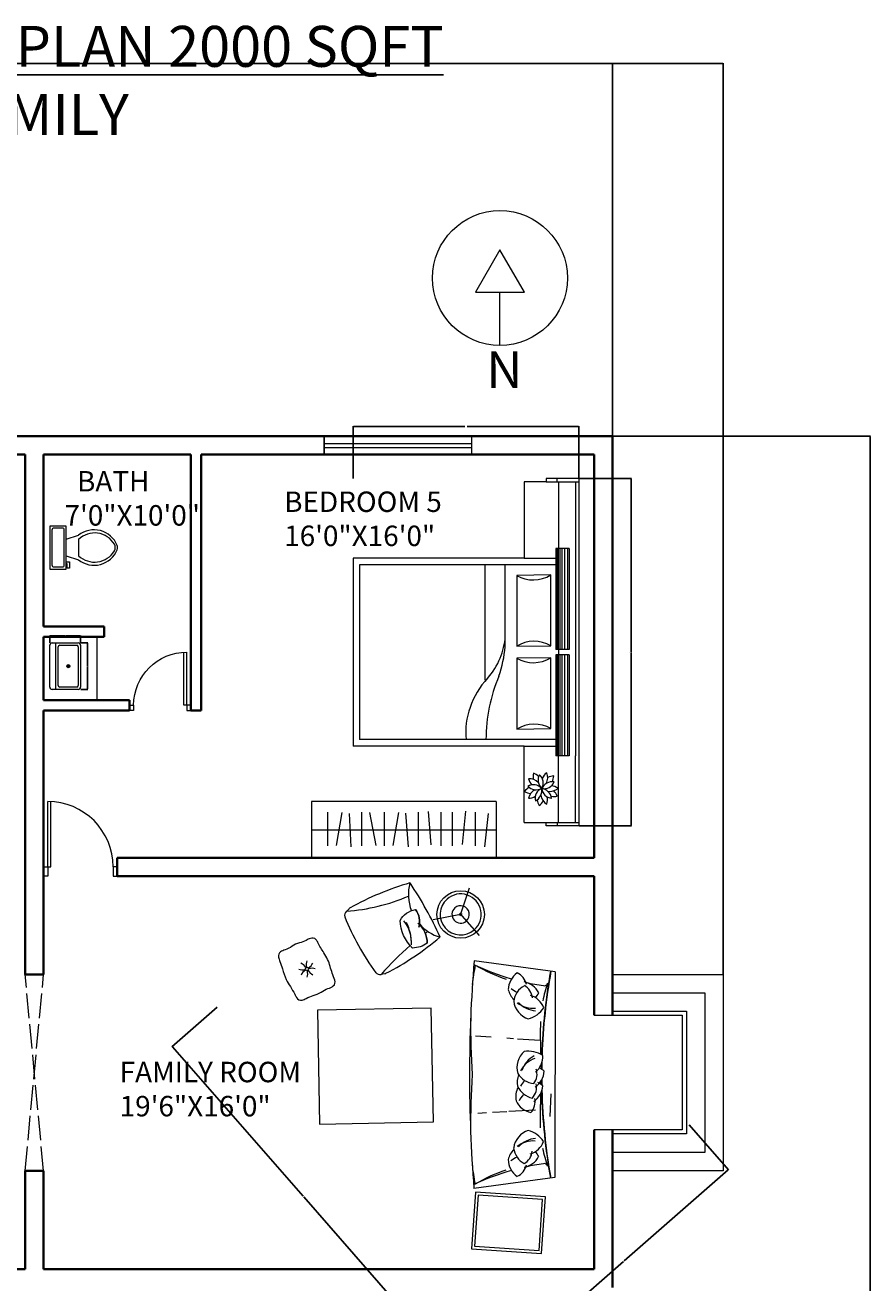
# Model space of a CAD drawing. Units: inches. Extents: x 4602 to 5612, y 5125 to 6591.
# Tile 6 of 6: x 5199 to 5612, y 5977 to 6591. Entities that reach past the tile are written whole.
import ezdxf

# ---------------------------------------------------------------- set-up
doc = ezdxf.new("R2010")
doc.units = ezdxf.units.IN
doc.linetypes.add('ACAD_ISO02W100', pattern=[15, 12, -3])
for name, color, linetype, lineweight in [('A-ANNO-DIMS', 2, 'Continuous', 18), ('A-ANNO-SYMB', 7, 'Continuous', 18), ('A-ANNO-TEXT', 7, 'Continuous', 25), ('A-AREA-IDEN', 7, 'Continuous', 18), ('A-DOOR', 4, 'Continuous', 18), ('A-FLOR-CASE', 9, 'Continuous', 18), ('A-FLOR-EDGE', 7, 'Continuous', 18), ('A-FLOR-FIXT', 8, 'Continuous', 18), ('A-FURN', 8, 'Continuous', 13), ('A-GLAZ', 4, 'Continuous', 18), ('A-WALL', 7, 'Continuous', 35), ('A-WALL-OVHD', 8, 'ACAD_ISO02W100', 13)]:
    doc.layers.add(name, color=color, linetype=linetype, lineweight=lineweight)
doc.styles.add('ATTR', font='romans.shx', dxfattribs={"width": 0.8, "height": 1.075})
doc.styles.get("Standard").update_dxf_attribs({"font": 'arial.ttf'})
doc.dimstyles.get("Standard").update_dxf_attribs({"dimtxt": 0.18, "dimasz": 0.18, "dimexe": 0.18, "dimexo": 0.0625, "dimgap": 0.09, "dimtad": 0, "dimtih": 1, "dimtoh": 1, "dimdec": 4, "dimzin": 0, "dimdsep": 46, "dimtxsty": 'Standard', "dimcen": 0.09, "dimadec": 0, "dimazin": 0, "dimtfac": 1, "dimtdec": 4, "dimtofl": 0, "dimtmove": 0, "dimatfit": 3, "dimfxl": 1, "dimtolj": 1, "dimtzin": 0, "dimarcsym": 0})

# ---------------------------------------------------------------- blocks, each defined once
blk = doc.blocks.new('A$C25213C04')
for p, q in [((2063, 2927, 1584), (1415, 2360, 1584)), ((2063, 2927, 1584), (3697, 1495, 1584)), ((961, 2561), (805, 2831)), ((961, 2590), (805, 2320)), ((936, 2575), (1248, 2575)), ((2506, 2330, 1584), (2338, 2162, 1584)), ((2306, 2131, 1584), (2256, 2081, 1584)), ((3178, 1881), (3005, 2048)), ((2140, 1966, 1584), (2022, 1849, 1584)), ((3026, 1811, 1584), (2854, 1589, 1584)), ((1493, 1691), (720, 773)), ((2411, 918), (1493, 1691)), ((2839, 1570, 1584), (2748, 1452, 1584)), ((3697, 1495, 1584), (3220, 778, 1584)), ((2708, 1401, 1584), (2653, 1329, 1584)), ((3783, 1288), (3260, 764)), ((3783, 1245), (3302, 764)), ((4207, 863), (3783, 1288)), ((4165, 863), (3783, 1245)), ((1638, 0), (2411, 918)), ((3684, 340), (4207, 863)), ((3684, 382), (4165, 863)), ((720, 773), (1638, 0)), ((3260, 764), (3684, 340)), ((3302, 764), (3684, 382))]:
    blk.add_line(p, q)
at = {"linetype": 'ByBlock'}
for p, q in [((133, 1730), (136, 1691)), ((896, 1561), (877, 1527))]:
    blk.add_line(p, q, dxfattribs=at)
blk.add_lwpolyline([(725, 2173, -0.232884), (950, 2110, -0.135002), (887, 1960, -0.190823), (579, 2053, -0.215879), (600, 2250, -0.243587), (764, 2155, 4.263709)], format="xyb")
blk.add_lwpolyline([(472, 697, 0.343499), (533, 723, 0.070096), (548, 767, -0.063818), (573, 843, 0.079553), (601, 928, -0.057815), (620, 1007, 0.080725), (637, 1068, 0.324043), (600, 1120, -0.019241), (459, 1179, 0.08432), (309, 1223, -0.023422), (183, 1248, 0.070372), (146, 1253, 0.295986), (100, 1217, 0.032258), (86, 1168, -0.067929), (60, 1097, 0.081366), (35, 1016, -0.070774), (15, 936, 0.059814), (0, 885, 0.300433), (27, 833, 0.039992), (72, 815, -0.020153), (147, 783, 0.038402), (259, 739, 0.019707), (344, 722, -0.015856), (435, 705, 0.018827), (472, 697, 1.060826)], format="xyb", dxfattribs=at)
at = {"linetype": 'ByBlock', "flags": 128}
blk.add_lwpolyline([(324, 993, -1), (314, 960, -1)], format="xyb", close=True, dxfattribs=at)
blk.add_circle((953, 2575), 250)
for centre, radius, start, end in [((6904, 6804, 1584), 6250, 218.7122, 226.8714), ((6904, 6804, 1584), 6246, 218.7173, 226.8972), ((2075, 2768, 1584), 34.6, 301.5027, 35.2471), ((3283, 3449, 1584), 1352, 209.2555, 217.5058), ((2065, 2440, 1584), 217, 75.8217, 128.2602), ((435, 4670, 1584), 2546, 306.4044, 310.6458), ((435, 4670, 1584), 2546, 293.2711, 302.9022), ((2031, 2594, 1584), 222, 173.7702, 227.3147), ((1881, 2465, 1584), 169, 60.105, 114.9918), ((2178, 2539, 1584), 222, 167.7702, 221.3147), ((2015, 2427, 1584), 169, 54.105, 108.9918), ((2196, 2383, 1584), 217, 69.8217, 122.2602), ((1856, 2548, 1584), 282, 8.7006, 21.3114), ((1999, 2512, 1584), 282, 333.4414, 15.3114), ((742, 2652), 470, 213.6928, 250.0667), ((-111, -1286), 3707, 72.7192, 82.835), ((908, 3983, 1584), 1733, 288.4557, 300.3041), ((1986, 2631, 1584), 226, 242.3583, 273.8129), ((1838, 2738, 1584), 282, 280.859, 296.2171), ((2136, 2581, 1584), 226, 236.3583, 300.7775), ((1993, 2688, 1584), 282, 280.859, 322.7291), ((2044, 2704, 1584), 282, 271.8903, 313.7604), ((7978, 8701, 1584), 8396, 227.9717, 230.3292), ((-1544, 2942), 2094, 323.3441, 341.8043), ((12303, 12967, 1584), 15201, 224.2521, 233.3075), ((3562, 3960, 1584), 2657, 217.5941, 222.0435), ((590, 2045), 206, 32.2825, 87.042), ((773, 1914), 264, 47.9991, 100.4376), ((742, 2652), 470, 270.1213, 301.8614), ((2720, 1975, 1584), 282, 105.7877, 147.6577), ((2708, 2129, 1584), 226, 180.3216, 244.7408), ((2862, 2114, 1584), 282, 167.3388, 209.2088), ((2874, 2061, 1584), 282, 158.3701, 200.2401), ((2508, 2077, 1584), 217, 358.839, 51.2774), ((6904, 6804, 1584), 6246, 227.5711, 228.2803), ((6904, 6804, 1584), 6250, 227.7194, 228.2519), ((7978, 8701, 1584), 8396, 231.1014, 231.3893), ((2825, 1872, 1584), 282, 99.7877, 112.3986), ((2625, 1995, 1584), 217, 352.839, 45.2774), ((591, 1710), 371, 44.935, 87.2084), ((487, 1559), 554, 48.4222, 73.8484), ((2639, 1946, 1584), 169, 12.1073, 66.9941), ((2930, 1759, 1584), 282, 99.7877, 112.3986), ((2741, 1851, 1584), 169, 6.1073, 60.9941), ((6904, 6804, 1584), 6246, 229.2463, 229.7871), ((6904, 6804, 1584), 6250, 229.3273, 229.7524), ((8643, 8118, 1584), 8396, 226.2108, 226.4615), ((2730, 1883, 1584), 217, 352.839, 45.2774), ((6904, 6804, 1584), 6246, 230.2513, 238.8423), ((10966, 12498, 1584), 13958, 229.1973, 231.6399), ((2651, 2143, 1584), 222, 259.7845, 313.329), ((2829, 2026, 1584), 226, 207.2862, 238.7408), ((2774, 2046, 1584), 222, 253.7845, 307.329), ((2997, 1955, 1584), 282, 184.882, 200.2401), ((6904, 6804, 1584), 6250, 230.3855, 238.8474), ((2846, 1738, 1584), 169, 6.1073, 60.9941), ((8643, 8118, 1584), 8396, 227.1305, 229.5879), ((2934, 1914, 1584), 226, 201.8609, 238.7408), ((2879, 1934, 1584), 222, 253.7845, 307.329), ((3102, 1842, 1584), 282, 184.882, 200.2401), ((3345, 1523, 1584), 226, 156.7821, 221.2013), ((3294, 1377, 1584), 282, 82.2482, 124.1182), ((3469, 1394, 1584), 282, 134.8306, 176.7006), ((3479, 1447, 1584), 282, 143.7993, 185.6693), ((3140, 1555, 1584), 217, 335.2995, 27.7379), ((4054, 2773, 1584), 1352, 240.0538, 248.3041), ((12014, 11580, 1584), 13958, 225.9197, 228.3623), ((3207, 1382, 1584), 169, 348.5678, 43.4546), ((3349, 1240, 1584), 282, 76.2482, 88.8591), ((3214, 1433, 1584), 217, 329.2995, 21.7379), ((5640, 111, 1584), 2546, 146.9138, 151.1553), ((3538, 1486, 1584), 34.6, 62.3126, 156.0569), ((3298, 1558, 1584), 222, 236.2449, 289.7895), ((3414, 1380, 1584), 226, 183.7467, 215.2013), ((3539, 1247, 1584), 282, 161.3425, 176.7006), ((3263, 1255, 1584), 169, 342.5678, 37.4546), ((5640, 111, 1584), 2546, 154.6574, 164.2885), ((3372, 1420, 1584), 222, 230.2449, 283.7895), ((4896, 489, 1584), 1733, 157.2556, 169.1039), ((4524, 3117, 1584), 2657, 235.5161, 239.9655)]:
    blk.add_arc(centre, radius, start, end)
at = {"linetype": 'ByBlock'}
for centre, radius, start, end in [((3117, 1104), 3051, 155.0292, 167.8975), ((4037, 1940), 3187, 175.3548, 175.9684), ((-2061, 2301), 3051, 346.2024, 359.1081), ((4037, 1940), 3187, 179.6641, 187.4345), ((168, 1736), 35.5, 167.4303, 189.0652), ((187, 1686), 51, 173.5933, 247.766), ((1112, 4418), 2936, 251.2253, 257.771), ((1098, 4417), 2932, 258.0523, 264.7029), ((826, 1556), 57.8, 270.4071, 330.8661), ((867, 1581), 35.5, 325.0347, 346.6697), ((215, 1016), 108, 350.0068, 26.3761), ((280, 872), 108, 80.0068, 116.3761), ((349, 1084), 108, 207.805, 244.1743), ((212, 1006), 108, 297.805, 334.1743), ((424, 937), 108, 170.0068, 206.3761), ((427, 947), 108, 117.805, 154.1743), ((290, 869), 108, 27.805, 64.1743), ((358, 1081), 108, 260.0068, 296.3761)]:
    blk.add_arc(centre, radius, start, end, dxfattribs=at)
for major_axis, start_param, end_param in [((-153, 153), 3.927057, 7.06865), ((-64.8, 64.8), 3.927057, 7.06865), ((-153, 153), 0.785465, 3.927057), ((-64.8, 64.8), 0.785465, 3.927057)]:
    blk.add_ellipse((953, 2575), major_axis=major_axis, ratio=1, start_param=start_param, end_param=end_param)
blk = doc.blocks.new("30'' Sink Single PV")
blk.add_line((-15, -3.999996), (15, -3.999996))
for points in [[(-13.5, 0), (13.5, 0)], [(-15, -18.499996), (-15, -1.5)], [(-13.5, -17.499996), (-13.5, -6.499996)], [(-12.5, -5.499996), (12.5, -5.499996)], [(13.5, -6.499996), (13.5, -17.499996)], [(15, -1.5), (15, -18.499996)], [(13.5, -19.999996), (-13.5, -19.999996)], [(12.5, -18.499996), (-12.5, -18.499996)]]:
    blk.add_lwpolyline(points)
for radius in [1, 0.5]:
    blk.add_circle((0, -11.999996), radius)
for centre, radius, start, end in [((-13.5, -1.5), 1.5, 90, 180), ((-12.5, -6.499996), 1, 90, 180), ((12.5, -6.499996), 1, 0, 90), ((13.5, -1.5), 1.5, 0, 90), ((-13.5, -18.499996), 1.5, 180, 270), ((-12.5, -17.499996), 1, 180, 270), ((12.5, -17.499996), 1, 270, 0), ((13.5, -18.499996), 1.5, 270, 0)]:
    blk.add_arc(centre, radius, start, end)
at = {"style": 'ATTR', "width": 0.8, "flags": 9}
blk.add_attdef('ESTCODE', (0, 0), '', height=0.006, dxfattribs=at)
blk = doc.blocks.new('A$C7BDD1693')
for p, q in [((0, 2.068), (0, 1.768)), ((0, 2.068), (1.615, 2.068)), ((0.03, 1.768), (0.03, 2.068)), ((0.03, 2.038), (0.64, 2.038)), ((0.64, 2.038), (1.565, 2.038)), ((0.64, 1.978), (1.565, 1.978)), ((0.64, 1.978), (0.64, 1.858)), ((0.64, 1.963), (1.565, 1.963)), ((1.565, 2.038), (1.615, 2.038)), ((1.565, 1.978), (1.565, 1.858)), ((1.615, 2.068), (2.54, 2.068)), ((1.615, 2.038), (2.54, 2.038)), ((1.615, 1.978), (1.615, 1.858)), ((1.615, 1.978), (2.54, 1.978)), ((1.615, 1.963), (2.54, 1.963)), ((2.54, 2.068), (3.18, 2.068)), ((3.15, 2.038), (2.54, 2.038)), ((2.54, 1.978), (2.54, 1.858)), ((3.15, 1.768), (3.15, 2.068)), ((3.18, 2.068), (3.18, 1.768)), ((0.03, 1.868), (0, 1.868)), ((0.03, 1.88), (0.64, 1.88)), ((0.64, 1.937), (1.565, 1.937)), ((0.64, 1.912), (1.565, 1.912)), ((0.64, 1.893), (1.565, 1.893)), ((0.64, 1.877), (1.565, 1.877)), ((0.64, 1.866), (1.565, 1.866)), ((0.64, 1.858), (1.565, 1.858)), ((0.73, 1.568), (0.73, 1.858)), ((0.79, 1.858), (0.79, 0.06)), ((1.565, 1.88), (1.615, 1.88)), ((1.615, 1.937), (2.54, 1.937)), ((1.615, 1.912), (2.54, 1.912)), ((1.615, 1.893), (2.54, 1.893)), ((1.615, 1.877), (2.54, 1.877)), ((1.615, 1.866), (2.54, 1.866)), ((1.615, 1.858), (2.54, 1.858)), ((2.39, 1.858), (2.39, 0.06)), ((2.45, 1.568), (2.45, 1.858)), ((3.15, 1.88), (2.54, 1.88)), ((3.15, 1.868), (3.18, 1.868)), ((0, 1.768), (0.03, 1.768)), ((0.03, 1.768), (0.03, 1.568)), ((0.03, 1.768), (0.03, 1.568)), ((1.533, 1.81), (0.883, 1.81)), ((0.883, 1.81), (0.887, 1.498)), ((1.537, 1.498), (1.533, 1.81)), ((2.291, 1.81), (1.641, 1.81)), ((1.641, 1.81), (1.646, 1.498)), ((2.296, 1.498), (2.291, 1.81)), ((3.15, 1.568), (3.15, 1.768)), ((3.18, 1.768), (3.15, 1.768)), ((0.03, 1.568), (0.73, 1.568)), ((0.73, 1.568), (0.73, 0)), ((0.887, 1.498), (1.537, 1.498)), ((1.646, 1.498), (2.296, 1.498)), ((3.15, 1.568), (2.45, 1.568)), ((2.45, 1.568), (2.45, 0)), ((1.54, 1.392), (0.79, 1.392)), ((1.848, 1.209), (0.79, 1.209)), ((0.73, 0), (2.45, 0)), ((0.79, 0.06), (2.39, 0.06))]:
    blk.add_line(p, q)
for centre, radius, start, end in [((2.938, 1.802), 0.125, 143.1301, 173.4932), ((2.751, 1.802), 0.115, 351.1324, 40.6013), ((2.967, 1.726), 0.155, 112.2105, 133.3514), ((2.817, 1.838), 0.0968, 345.5086, 19.2476), ((0.626, 1.65), 0.303, 329.8722, 31.8713), ((1.794, 1.658), 0.303, 149.8722, 211.8713), ((1.384, 1.65), 0.303, 329.8722, 31.8713), ((2.553, 1.658), 0.303, 149.8722, 211.8713), ((2.74, 1.667), 0.115, 63.1324, 112.6013), ((2.798, 1.845), 0.125, 215.1301, 245.4931), ((2.788, 1.643), 0.098, 59.0447, 140.2473), ((2.879, 1.849), 0.155, 184.2105, 205.3514), ((2.726, 1.74), 0.0968, 57.5086, 91.2476), ((2.884, 1.823), 0.106, 170.7761, 244.5159), ((2.743, 1.749), 0.098, 347.0447, 68.2473), ((2.944, 1.713), 0.106, 98.7761, 172.5159), ((2.83, 1.825), 0.098, 275.0447, 356.2473), ((2.858, 1.622), 0.106, 26.7761, 100.5159), ((2.883, 1.833), 0.115, 279.1324, 328.6013), ((2.941, 1.655), 0.125, 71.1301, 101.4931), ((2.877, 1.605), 0.155, 40.2105, 61.3514), ((2.791, 1.624), 0.0968, 129.5086, 163.2476), ((2.735, 1.803), 0.155, 256.2105, 277.3514), ((2.761, 1.8), 0.106, 242.7761, 316.5159), ((2.865, 1.615), 0.115, 135.1324, 184.6013), ((2.713, 1.725), 0.125, 287.1301, 317.4932), ((2.903, 1.653), 0.098, 131.0447, 212.2473), ((2.745, 1.676), 0.106, 314.7761, 28.5159), ((2.921, 1.65), 0.0968, 201.5086, 235.2476), ((2.929, 1.765), 0.098, 203.0447, 284.2473), ((2.953, 1.718), 0.115, 207.1324, 256.6013), ((2.734, 1.652), 0.155, 328.2105, 349.3514), ((2.802, 1.607), 0.125, 359.1301, 29.4932), ((2.937, 1.782), 0.0968, 273.5086, 307.2476)]:
    blk.add_arc(centre, radius, start, end)
for centre, major_axis, ratio, start_param, end_param in [((1.413, 0.552), (0, -0.842), 0.84, 2.512571, 3.097265), ((1.474, 0.023), (0, -1.371), 0.84, 2.845884, 3.083884), ((2.394, 3.329), (0, -2.112), 0.84, -0.336035, -0.002349), ((2.261, 1.856), (0.259, -0.793), 0.868451, -0.988378, -0.183496)]:
    blk.add_ellipse(centre, major_axis=major_axis, ratio=ratio, start_param=start_param, end_param=end_param)
blk = doc.blocks.new('*U9')
for p, q in [((241, -152), (241, -51)), ((-254, -216), (-203, -216)), ((-254, -241), (-254, -216)), ((-178, -241), (-254, -241)), ((-203, -216), (-203, -203)), ((-178, -203), (-178, -241)), ((-102, -203), (-152, -356)), ((102, -203), (152, -356)), ((102, -356), (-102, -356))]:
    blk.add_line(p, q)
blk.add_lwpolyline([(267, -203), (267, 0), (-267, 0), (-267, -203)], close=True)
for points in [[(-241, -51), (-241, -152)], [(216, -25), (-216, -25)], [(-216, -178), (216, -178)]]:
    blk.add_lwpolyline(points)
for centre, radius, start, end in [((-219, -48), 22.5, 81.8699, 188.1301), ((-219, -156), 22.5, 171.8699, 278.1301), ((219, -48), 22.5, 351.8699, 98.1301), ((219, -156), 22.5, 261.8699, 8.1301), ((89, -548), 309, 141.4691, 247.9714), ((107, -554), 288, 136.3677, 238.9468), ((-89, -548), 309, 292.0284, 38.5307), ((-107, -554), 288, 301.053, 43.6321), ((0, -708), 102, 245.7318, 294.2682), ((0, -737), 102, 254.8605, 285.1395)]:
    blk.add_arc(centre, radius, start, end)
blk = doc.blocks.new('DOOR-36IN-DEEP-JAMB')
for p, q in [((2, 4.5), (2, 36.5)), ((3.5, 4.5), (3.5, 36.46)), ((0, 4.5), (2, 4.5)), ((2, 4.5), (2, 0)), ((2, 4.5), (3.5, 4.5)), ((36, 4.5), (34, 4.5)), ((34, 4.5), (34, 0)), ((2, 0), (0, 0)), ((34, 0), (36, 0))]:
    blk.add_line(p, q)
blk.add_arc((2, 4.5), 32, 0, 90)
blk = doc.blocks.new('DOOR-30IN')
for p, q in [((26, 30), (26, 28)), ((26, 28), (28.5, 28)), ((28.5, 28), (28.5, 30)), ((26, 2), (0, 2)), ((26, 3.5), (0.04, 3.5)), ((26, 2), (26, 3.5)), ((26, 0), (26, 2)), ((26, 2), (28.5, 2)), ((28.5, 2), (28.5, 0))]:
    blk.add_line(p, q)
blk.add_arc((26, 2), 26, 90, 180)
blk = doc.blocks.new('WINDOW-72IN')
for p, q in [((9, 72), (0, 72)), ((3.5, 72), (3.5, 0)), ((5.5, 72), (5.5, 0)), ((9, 0), (0, 0))]:
    blk.add_line(p, q)
blk = doc.blocks.new('WARDROBE-RAIL')
for p, q in [((90.22, 0), (90.22, 27.46)), ((3.99, 5.88), (5.71, 22.16)), ((10.39, 5.25), (10.39, 21.62)), ((15.01, 4.71), (16.73, 21)), ((21.48, 5.25), (21.48, 21.62)), ((27.02, 5.25), (27.02, 21.62)), ((33.26, 4.83), (31.94, 21.15)), ((38.1, 5.25), (38.1, 21.62)), ((44.31, 5.72), (42.98, 22.05)), ((47.72, 5.36), (50.53, 21.49)), ((54.72, 5.25), (54.72, 21.62)), ((61.87, 5.4), (58.77, 21.48)), ((65.8, 5.25), (65.8, 21.62)), ((70.89, 22.2), (71.76, 5.85)), ((75.49, 5.36), (78.19, 21.52)), ((82.43, 5.25), (82.43, 21.62)), ((90.22, 13.73), (0, 13.73)), ((0, 0), (90.22, 0))]:
    blk.add_line(p, q)
blk = doc.blocks.new('*D33')
at = {"layer": 'A-ANNO-DIMS', "color": 0, "lineweight": -2, "transparency": 16777216}
for p, q in [((5469.82, 6369.91), (5495.4, 6369.91)), ((5495.22, 6369.73), (5495.22, 6285.24)), ((5495.22, 6200.39), (5495.22, 6284.88)), ((5469.82, 6200.21), (5495.4, 6200.21))]:
    blk.add_line(p, q, dxfattribs=at)
at = {"layer": 'A-ANNO-DIMS', "color": 0, "transparency": 16777216}
for points in [[(5495.19, 6369.73), (5495.25, 6369.73), (5495.22, 6369.91)], [(5495.19, 6200.39), (5495.25, 6200.39), (5495.22, 6200.21)]]:
    blk.add_solid(points, dxfattribs=at)
at = {"layer": 'Defpoints', "color": 0, "transparency": 16777216}
for p in [(5469.76, 6369.91), (5469.76, 6200.21), (5495.22, 6200.21)]:
    blk.add_point(p, dxfattribs=at)
at = {"layer": 'A-ANNO-DIMS', "color": 0, "transparency": 16777216, "insert": (5495.22, 6285.06), "char_height": 0.18, "attachment_point": 5}
blk.add_mtext('\\A1;BED GROUP 170 TYP.', dxfattribs=at)
blk = doc.blocks.new('*D34')
at = {"layer": 'A-ANNO-DIMS', "color": 0, "lineweight": -2, "transparency": 16777216}
for p, q in [((5359.4, 6369.97), (5359.4, 6395.55)), ((5359.58, 6395.37), (5413.99, 6395.37)), ((5469.58, 6395.37), (5415.17, 6395.37)), ((5469.76, 6369.97), (5469.76, 6395.55))]:
    blk.add_line(p, q, dxfattribs=at)
at = {"layer": 'A-ANNO-DIMS', "color": 0, "transparency": 16777216}
for points in [[(5359.58, 6395.4), (5359.58, 6395.34), (5359.4, 6395.37)], [(5469.58, 6395.4), (5469.58, 6395.34), (5469.76, 6395.37)]]:
    blk.add_solid(points, dxfattribs=at)
at = {"layer": 'Defpoints', "color": 0, "transparency": 16777216}
for p in [(5469.76, 6395.37), (5359.4, 6369.91), (5469.76, 6369.91)]:
    blk.add_point(p, dxfattribs=at)
at = {"layer": 'A-ANNO-DIMS', "color": 0, "transparency": 16777216, "insert": (5414.58, 6395.37), "char_height": 0.18, "attachment_point": 5}
blk.add_mtext('\\A1;110 TYP.', dxfattribs=at)
blk = doc.blocks.new('*D41')
at = {"layer": 'A-ANNO-DIMS', "color": 0, "lineweight": -2, "transparency": 16777216}
for p, q in [((5226.4, 6289.53), (5229.92, 6289.53)), ((5229.74, 6289.35), (5229.74, 6278.37)), ((5229.74, 6267.03), (5229.74, 6278)), ((5226.4, 6266.85), (5229.92, 6266.85))]:
    blk.add_line(p, q, dxfattribs=at)
at = {"layer": 'A-ANNO-DIMS', "color": 0, "transparency": 16777216}
for points in [[(5229.71, 6289.35), (5229.77, 6289.35), (5229.74, 6289.53)], [(5229.71, 6267.03), (5229.77, 6267.03), (5229.74, 6266.85)]]:
    blk.add_solid(points, dxfattribs=at)
at = {"layer": 'Defpoints', "color": 0, "transparency": 16777216}
for p in [(5226.34, 6289.53), (5229.74, 6289.53), (5226.34, 6266.85)]:
    blk.add_point(p, dxfattribs=at)
at = {"layer": 'A-ANNO-DIMS', "color": 0, "transparency": 16777216, "insert": (5229.74, 6278.19), "char_height": 0.18, "attachment_point": 5}
blk.add_mtext('\\A1;BASIN 23', dxfattribs=at)
blk = doc.blocks.new('*D42')
at = {"layer": 'A-ANNO-DIMS', "color": 0, "lineweight": -2, "transparency": 16777216}
for p, q in [((5211.21, 6289.59), (5211.21, 6293.11)), ((5211.39, 6292.93), (5218.56, 6292.93)), ((5226.16, 6292.93), (5218.99, 6292.93)), ((5226.34, 6289.59), (5226.34, 6293.11))]:
    blk.add_line(p, q, dxfattribs=at)
at = {"layer": 'A-ANNO-DIMS', "color": 0, "transparency": 16777216}
for points in [[(5211.39, 6292.96), (5211.39, 6292.9), (5211.21, 6292.93)], [(5226.16, 6292.96), (5226.16, 6292.9), (5226.34, 6292.93)]]:
    blk.add_solid(points, dxfattribs=at)
at = {"layer": 'Defpoints', "color": 0, "transparency": 16777216}
for p in [(5211.21, 6292.93), (5211.21, 6289.53), (5226.34, 6289.53)]:
    blk.add_point(p, dxfattribs=at)
at = {"layer": 'A-ANNO-DIMS', "color": 0, "transparency": 16777216, "insert": (5218.78, 6292.93), "char_height": 0.18, "attachment_point": 5}
blk.add_mtext('\\A1;15', dxfattribs=at)
blk = doc.blocks.new('*D49')
at = {"layer": 'A-ANNO-DIMS', "color": 0, "lineweight": -2, "transparency": 16777216}
for p, q in [((5293.01, 6111.54), (5270.91, 6092.21)), ((5271.16, 6092.19), (5335.08, 6019.13)), ((5399.32, 5945.7), (5335.4, 6018.76)), ((5421.4, 5964.78), (5399.3, 5945.45))]:
    blk.add_line(p, q, dxfattribs=at)
at = {"layer": 'A-ANNO-DIMS', "color": 0, "transparency": 16777216}
for points in [[(5271.18, 6092.21), (5271.14, 6092.17), (5271.04, 6092.33)], [(5399.34, 5945.72), (5399.29, 5945.68), (5399.43, 5945.57)]]:
    blk.add_solid(points, dxfattribs=at)
at = {"layer": 'Defpoints', "color": 0, "transparency": 16777216}
for p in [(5293.05, 6111.58), (5421.45, 5964.83), (5399.43, 5945.57)]:
    blk.add_point(p, dxfattribs=at)
at = {"layer": 'A-ANNO-DIMS', "color": 0, "transparency": 16777216, "insert": (5335.24, 6018.95), "char_height": 0.18, "attachment_point": 5}
blk.add_mtext('\\A1;FAMILY SEATING 195', dxfattribs=at)
blk = doc.blocks.new('*D50')
at = {"layer": 'A-ANNO-DIMS', "color": 0, "lineweight": -2, "transparency": 16777216}
for p, q in [((5523.54, 6054.06), (5542.88, 6031.96)), ((5542.62, 6031.97), (5491.94, 5987.63)), ((5440.84, 5942.93), (5491.53, 5987.27)), ((5421.49, 5964.78), (5440.83, 5942.68))]:
    blk.add_line(p, q, dxfattribs=at)
at = {"layer": 'A-ANNO-DIMS', "color": 0, "transparency": 16777216}
for points in [[(5542.6, 6032), (5542.64, 6031.95), (5542.76, 6032.09)], [(5440.82, 5942.95), (5440.86, 5942.91), (5440.71, 5942.81)]]:
    blk.add_solid(points, dxfattribs=at)
at = {"layer": 'Defpoints', "color": 0, "transparency": 16777216}
for p in [(5523.5, 6054.11), (5542.76, 6032.09), (5421.45, 5964.83)]:
    blk.add_point(p, dxfattribs=at)
at = {"layer": 'A-ANNO-DIMS', "color": 0, "transparency": 16777216, "insert": (5491.73, 5987.45), "char_height": 0.18, "attachment_point": 5}
blk.add_mtext('\\A1;136', dxfattribs=at)
blk = doc.blocks.new('*D55')
at = {"layer": 'A-ANNO-DIMS', "color": 0, "lineweight": -2, "transparency": 16777216}
for p, q in [((4674.24, 6252.95), (4674.24, 6572.85)), ((4674.42, 6572.67), (5106.95, 6572.67)), ((5540.06, 6572.67), (5107.53, 6572.67)), ((5540.24, 6127.61), (5540.24, 6572.85))]:
    blk.add_line(p, q, dxfattribs=at)
at = {"layer": 'A-ANNO-DIMS', "color": 0, "transparency": 16777216}
for points in [[(4674.42, 6572.7), (4674.42, 6572.64), (4674.24, 6572.67)], [(5540.06, 6572.7), (5540.06, 6572.64), (5540.24, 6572.67)]]:
    blk.add_solid(points, dxfattribs=at)
at = {"layer": 'Defpoints', "color": 0, "transparency": 16777216}
for p in [(5540.24, 6572.67), (4674.24, 6252.89), (5540.24, 6127.55)]:
    blk.add_point(p, dxfattribs=at)
at = {"layer": 'A-ANNO-DIMS', "color": 0, "transparency": 16777216, "insert": (5107.24, 6572.67), "char_height": 0.18, "attachment_point": 5}
blk.add_mtext('\\A1;866', dxfattribs=at)
blk = doc.blocks.new('*D58')
at = {"layer": 'A-ANNO-DIMS', "color": 0, "lineweight": -2, "transparency": 16777216}
for p, q in [((5486.3, 6390.55), (5612.27, 6390.55)), ((5612.09, 6390.37), (5612.09, 5885.73)), ((5612.09, 5380.73), (5612.09, 5885.37)), ((5486.3, 5380.55), (5612.27, 5380.55))]:
    blk.add_line(p, q, dxfattribs=at)
at = {"layer": 'A-ANNO-DIMS', "color": 0, "transparency": 16777216}
for points in [[(5612.06, 6390.37), (5612.12, 6390.37), (5612.09, 6390.55)], [(5612.06, 5380.73), (5612.12, 5380.73), (5612.09, 5380.55)]]:
    blk.add_solid(points, dxfattribs=at)
at = {"layer": 'Defpoints', "color": 0, "transparency": 16777216}
for p in [(5486.24, 6390.55), (5612.09, 6390.55), (5486.24, 5380.55)]:
    blk.add_point(p, dxfattribs=at)
at = {"layer": 'A-ANNO-DIMS', "color": 0, "transparency": 16777216, "insert": (5612.09, 5885.55), "char_height": 0.18, "attachment_point": 5}
blk.add_mtext('\\A1;1010', dxfattribs=at)
blk = doc.blocks.new('*D70')
at = {"layer": 'A-ANNO-DIMS', "color": 0, "lineweight": -2, "transparency": 16777216}
for p, q in [((5486.24, 6127.61), (5486.24, 6572.85)), ((5486.42, 6572.67), (5513.02, 6572.67)), ((5540.06, 6572.67), (5513.46, 6572.67)), ((5540.24, 6127.61), (5540.24, 6572.85))]:
    blk.add_line(p, q, dxfattribs=at)
at = {"layer": 'A-ANNO-DIMS', "color": 0, "transparency": 16777216}
for points in [[(5486.42, 6572.7), (5486.42, 6572.64), (5486.24, 6572.67)], [(5540.06, 6572.7), (5540.06, 6572.64), (5540.24, 6572.67)]]:
    blk.add_solid(points, dxfattribs=at)
at = {"layer": 'Defpoints', "color": 0, "transparency": 16777216}
for p in [(5540.24, 6572.67), (5486.24, 6127.55), (5540.24, 6127.55)]:
    blk.add_point(p, dxfattribs=at)
at = {"layer": 'A-ANNO-DIMS', "color": 0, "transparency": 16777216, "insert": (5513.24, 6572.67), "char_height": 0.18, "attachment_point": 5}
blk.add_mtext('\\A1;54', dxfattribs=at)

msp = doc.modelspace()

# ---------------------------------------------------------------- linework, layer by layer
at = {"layer": 'A-ANNO-SYMB'}
msp.add_line((5431.1739, 6434.9332), (5431.1739, 6460.9693), dxfattribs=at)
msp.add_lwpolyline([(5431.1739, 6481.6935), (5419.2088, 6460.9693), (5443.1391, 6460.9693)], close=True, dxfattribs=at)
msp.add_circle((5431.1739, 6467.8774), 32.9442, dxfattribs=at)
at = {"layer": 'A-FLOR-CASE'}
for p, q in [((5234.1748, 6292.5515), (5234.1748, 6261.5515)), ((5429.3878, 6212.0089), (5429.3878, 6184.5515))]:
    msp.add_line(p, q, dxfattribs=at)
at = {"layer": 'A-FLOR-EDGE'}
for p, q in [((5486.239, 6127.5515), (5540.239, 6127.5515)), ((5540.239, 6127.5515), (5540.239, 6031.5515)), ((5486.239, 6118.5515), (5531.239, 6118.5515)), ((5531.239, 6118.5515), (5531.239, 6040.5515)), ((5477.239, 6107.5515), (5520.239, 6107.5515)), ((5486.239, 6109.5515), (5522.239, 6109.5515)), ((5520.239, 6107.5515), (5520.239, 6051.5515)), ((5522.239, 6109.5515), (5522.239, 6049.5515)), ((5520.239, 6051.5515), (5477.239, 6051.5515)), ((5522.239, 6049.5515), (5486.239, 6049.5515)), ((5531.239, 6040.5515), (5486.239, 6040.5515)), ((5540.239, 6031.5515), (5486.239, 6031.5515))]:
    msp.add_line(p, q, dxfattribs=at)
at = {"layer": 'A-GLAZ'}
msp.add_line((5345.239, 6381.5515), (5345.239, 6390.5515), dxfattribs=at)
at = {"layer": 'A-WALL'}
for p, q in [((5133.239, 6390.5515), (5486.239, 6390.5515)), ((5486.239, 6390.5515), (5486.239, 6175.5515)), ((5133.239, 6381.5515), (5199.239, 6381.5515)), ((5199.239, 6381.5515), (5199.239, 6127.5515)), ((5208.239, 6381.5515), (5208.239, 6297.5515)), ((5208.239, 6381.5515), (5280.239, 6381.5515)), ((5280.239, 6381.5515), (5280.239, 6256.5515)), ((5285.239, 6381.5515), (5285.239, 6256.5515)), ((5285.239, 6381.5515), (5477.239, 6381.5515)), ((5477.239, 6381.5515), (5477.239, 6184.5515)), ((5208.239, 6297.5515), (5237.8576, 6297.5515)), ((5237.8576, 6292.5515), (5237.8576, 6297.5515)), ((5208.239, 6292.5515), (5237.8576, 6292.5515)), ((5208.239, 6292.5515), (5208.239, 6261.5515)), ((5208.239, 6261.5515), (5250.239, 6261.5515)), ((5250.239, 6261.5515), (5250.239, 6256.5515)), ((5208.239, 6256.5515), (5250.239, 6256.5515)), ((5208.239, 6256.5515), (5208.239, 6127.5515)), ((5280.239, 6256.5515), (5285.239, 6256.5515)), ((5477.239, 6184.5515), (5244.239, 6184.5515)), ((5244.239, 6184.5515), (5244.239, 6175.5515)), ((5477.239, 6175.5515), (5244.239, 6175.5515)), ((5477.239, 6175.5515), (5477.239, 6107.5515)), ((5486.239, 6175.5515), (5486.239, 6107.5515)), ((5208.239, 6127.5515), (5199.239, 6127.5515)), ((5477.239, 6051.5515), (5477.239, 5983.5515)), ((5486.239, 6051.5515), (5486.239, 5974.5515)), ((5199.239, 6031.5515), (5199.239, 5983.5515)), ((5208.239, 6031.5515), (5199.239, 6031.5515)), ((5208.239, 6031.5515), (5208.239, 5983.5515)), ((5199.239, 5983.5515), (5110.739, 5983.5515)), ((5477.239, 5983.5515), (5208.239, 5983.5515))]:
    msp.add_line(p, q, dxfattribs=at)
at = {"layer": 'A-WALL-OVHD'}
for p, q in [((5199.239, 6031.5515), (5208.239, 6127.5515)), ((5208.239, 6031.5515), (5199.239, 6127.5515))]:
    msp.add_line(p, q, dxfattribs=at)

# ---------------------------------------------------------------- block references
at = {"layer": 'A-DOOR', "extrusion": (0, 0, -1), "zscale": -1, "rotation": 269.9999999999923}
msp.add_blockref('DOOR-30IN', (-5280.2386, 6285.0516), dxfattribs=at)
at = {"layer": 'A-DOOR'}
msp.add_blockref('DOOR-36IN-DEEP-JAMB', (5208.239, 6175.552), dxfattribs=at)
at = {"layer": 'A-FLOR-CASE', "rotation": 180}
msp.add_blockref('WARDROBE-RAIL', (5429.3878, 6212.009), dxfattribs=at)
at = {"layer": 'A-FLOR-FIXT', "rotation": 90}
for name, p, xscale, yscale, zscale in [('*U9', (5211.3349, 6336.1611), 0.0393700787401575, 0.0393700787401575, 0.0393700787401575), ("30'' Sink Single PV", (5211.2171, 6278.1873), 0.7560519261215212, 0.7560519261215212, 0.7560519261215212)]:
    msp.add_blockref(name, p, dxfattribs=dict(at, xscale=xscale, yscale=yscale, zscale=zscale))
at = {"layer": 'A-FURN'}
for name, p, xscale, yscale, zscale, rotation in [('A$C7BDD1693', (5359.4042, 6369.9111), 53.36654952143724, 53.36654952143724, 53.36654952143724, 270), ('A$C25213C04', (5293.1099, 6111.5215, -73.3869), 0.0463301076927589, 0.0463301076927589, 0.0463301076927589, 311.1814570076615)]:
    msp.add_blockref(name, p, dxfattribs=dict(at, xscale=xscale, yscale=yscale, zscale=zscale, rotation=rotation))
at = {"layer": 'A-GLAZ', "rotation": 90.00000000000003}
msp.add_blockref('WINDOW-72IN', (5417.2386, 6381.5515), dxfattribs=at)

# ---------------------------------------------------------------- texts
at = {"layer": 'A-ANNO-SYMB', "insert": (5424.4632, 6432.0953), "char_height": 18, "attachment_point": 1}
msp.add_mtext_dynamic_manual_height_columns('N', width=25.525886, gutter_width=12.5, heights=[0], dxfattribs=at)
at = {"layer": 'A-ANNO-TEXT', "insert": (4812.35, 6591.1079), "char_height": 20, "attachment_point": 1}
msp.add_mtext_dynamic_manual_height_columns('{\\LKERALA TRADITIONAL HOUSE PLAN 2000 SQFT \\P}      DESIGNED FOR A LARGE FAMILY\\P              {\\LGROUND FLOOR PLAN}', width=869.722344, gutter_width=12.5, heights=[0], dxfattribs=at)
at = {"layer": 'A-AREA-IDEN', "char_height": 10, "attachment_point": 1}
for s, width, insert in [('  BATH \\P7\'0"X10\'0"', 127.373556, (5218.4592, 6373.5514)), ('BEDROOM 5\\P16\'0"X16\'0"', 161.964905, (5325.7719, 6363.5446)), ('FAMILY ROOM\\P19\'6"X16\'0"', 326.752228, (5245.4089, 6084.8361))]:
    msp.add_mtext_dynamic_manual_height_columns(s, width=width, gutter_width=12.5, heights=[0], dxfattribs=dict(at, insert=insert))

# ---------------------------------------------------------------- dimensions: what is measured, and where the dimension line sits
at = {"layer": 'A-ANNO-DIMS'}
for p1, picture, middle in [((4674.239, 6252.8852), '*D55', (5107.239, 6572.6716)), ((5486.239, 6127.5515), '*D70', (5513.239, 6572.6716))]:
    dim = msp.add_linear_dim(base=(5540.239, 6572.6716), p1=p1, p2=(5540.239, 6127.5515), dimstyle='Standard', override={"dimdec": 0, "dimlfac": 1, "dimrnd": 0, "dimzin": 0, "dimdsep": 46, "dimlunit": 2}, dxfattribs=at)
    dim.commit()
    dim.dimension.update_dxf_attribs({"geometry": picture, "text_midpoint": middle})
dim = msp.add_linear_dim(base=(5469.7601, 6395.3669), p1=(5359.4042, 6369.9111), p2=(5469.7601, 6369.9111), text='<> TYP.', dimstyle='Standard', override={"dimdec": 0, "dimlfac": 1, "dimrnd": 0, "dimzin": 0, "dimdsep": 46, "dimlunit": 2}, dxfattribs=at)
dim.commit()
dim.dimension.update_dxf_attribs({"geometry": '*D34', "text_midpoint": (5414.5822, 6395.3669)})
for base, p1, p2, angle, picture, middle in [((5612.089, 6390.5515), (5486.239, 5380.5515), (5486.239, 6390.5515), 90, '*D58', (5612.089, 5885.5515)), ((5211.2125, 6292.9303), (5226.3381, 6289.5281), (5211.2125, 6289.5281), 180, '*D42', (5218.7753, 6292.9303)), ((5542.7583, 6032.0917), (5421.4487, 5964.8254), (5523.4992, 6054.1055), 41.181457, '*D50', (5491.7331, 5987.4516))]:
    dim = msp.add_linear_dim(base=base, p1=p1, p2=p2, angle=angle, dimstyle='Standard', override={"dimdec": 0, "dimlfac": 1, "dimrnd": 0, "dimzin": 0, "dimdsep": 46, "dimlunit": 2}, dxfattribs=at)
    dim.commit()
    dim.dimension.update_dxf_attribs({"geometry": picture, "text_midpoint": middle})
for base, p1, p2, angle, text, picture, middle in [((5495.216, 6200.2055), (5469.7601, 6369.9111), (5469.7601, 6200.2055), 270, 'BED GROUP <> TYP.', '*D33', (5495.216, 6285.0583)), ((5229.7403, 6289.5281), (5226.3381, 6266.8465), (5226.3381, 6289.5281), 90, 'BASIN <>', '*D41', (5229.7403, 6278.1873)), ((5399.4348, 5945.5663), (5293.0546, 6111.5847), (5421.4487, 5964.8254), 311.181457, 'FAMILY SEATING <>', '*D49', (5335.2378, 6018.9459))]:
    dim = msp.add_linear_dim(base=base, p1=p1, p2=p2, angle=angle, text=text, dimstyle='Standard', override={"dimdec": 0, "dimlfac": 1, "dimrnd": 0, "dimzin": 0, "dimdsep": 46, "dimlunit": 2}, dxfattribs=at)
    dim.commit()
    dim.dimension.update_dxf_attribs({"geometry": picture, "text_midpoint": middle})

doc.saveas('drawing.dxf')
